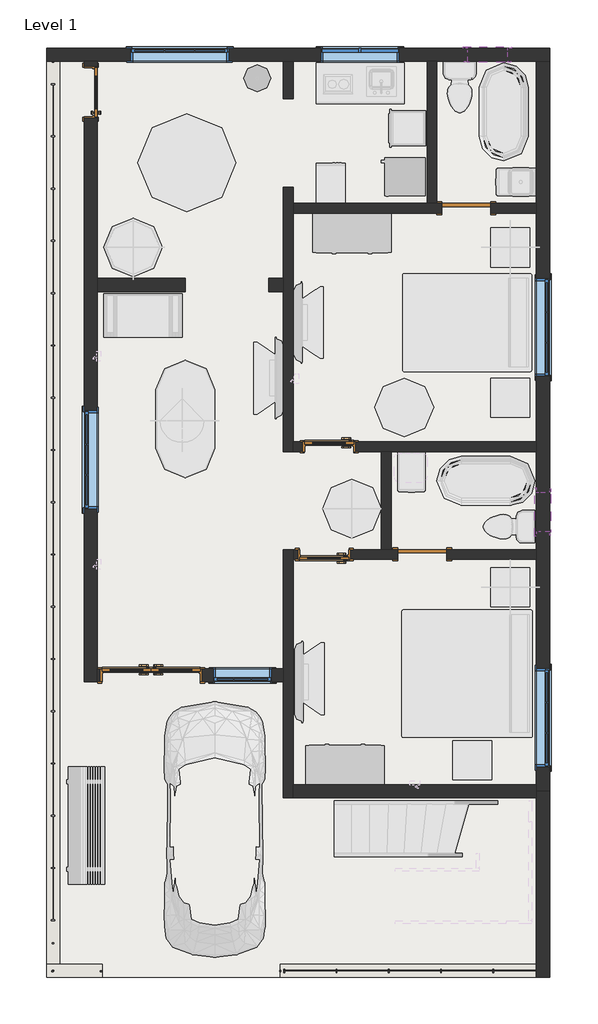
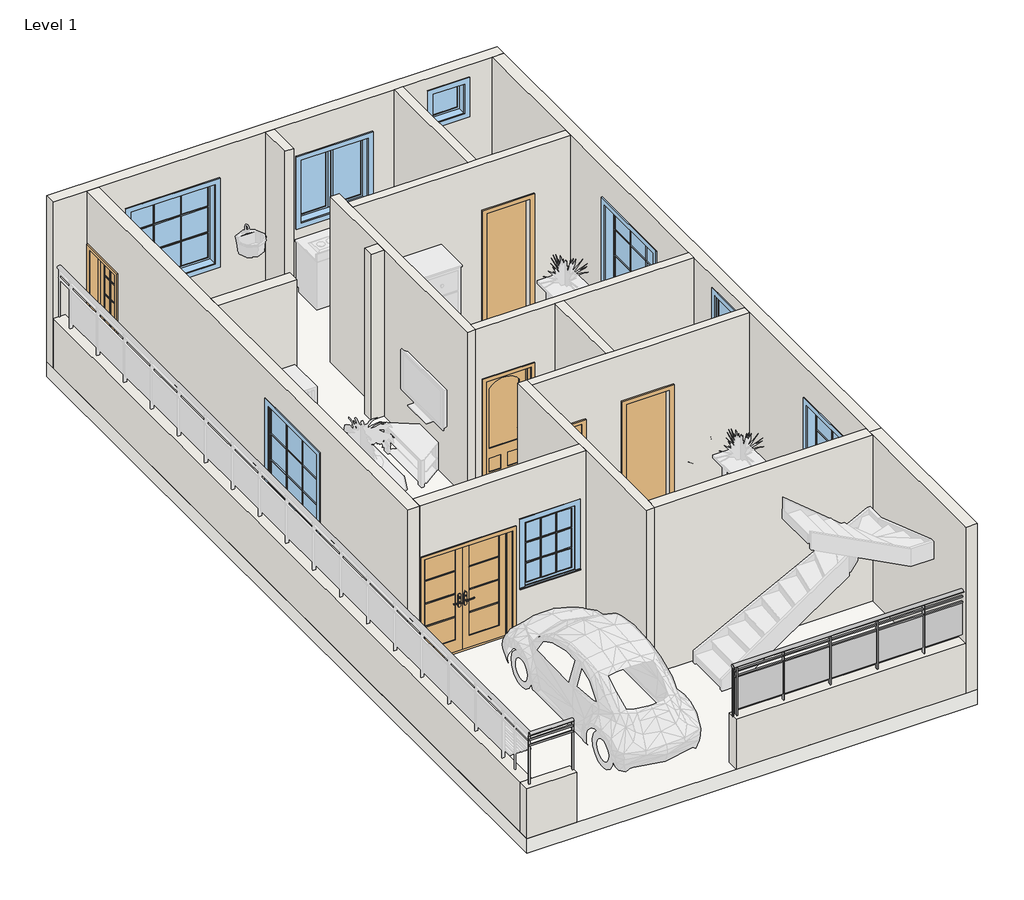
# One storey, part 1 of 2: 19 walls, 8 windows, 6 doors, 2 railings, 1 slab.
"""IFC4 building model written with IfcOpenShell, lengths in millimetres."""

from ifc_helpers import new_model, si_unit, point, frame, origin, origin_with_axes, place, context, project, spatial, polyline, ellipse_curve, trimmed, outline, extrude, faceted_brep, transform, mapped, element, save
from ifc_brep_helpers import plane_surface, extruded_surface, advanced_brep
from components import door_4b146b56, door_14b9be53, door_b03bd389, door_d788789e, door_e2b13fe9, window_29c06734, window_8901c6e2, window_0862ab64, window_e41d21a6

model = new_model("IFC4")

# Units and contexts
model_context = context("Model", 3, world=origin())
ifc_project = project(units=[si_unit("LENGTHUNIT", "METRE", prefix="MILLI")], contexts=[model_context])

# Site, building, storey
site = spatial("IfcSite", under=ifc_project)
building = spatial("IfcBuilding", under=site)
storey = spatial("IfcBuildingStorey", under=building, Name="Level 1", Elevation=0.0)

# Doors
placement = place(None, origin())
door_shape = door_4b146b56(model_context)
element("IfcDoor", 1, ObjectType="30\" x 80\"", at=placement, inside=storey, context=model_context, shape_type="MappedRepresentation", body=[
    mapped(door_shape, transform((-1899.3247449, 6788.0508877, 0.0), x_axis=(1.0, 0.0, 0.0), y_axis=(0.0, 1.0, 0.0), z_axis=(0.0, 0.0, 1.0))),
])
door_2_shape = door_14b9be53(model_context)
element("IfcDoor", 2, ObjectType="30\" x 80\"", at=placement, inside=storey, context=model_context, shape_type="MappedRepresentation", body=[
    mapped(door_2_shape, transform((-1823.1247449, 8470.8008877, 0.0), x_axis=(1.0, 0.0, 0.0), y_axis=(0.0, 1.0, 0.0), z_axis=(0.0, 0.0, 1.0))),
])
door_3_shape = door_b03bd389(model_context)
element("IfcDoor", 3, ObjectType="Door-Exterior-Double-Full Glass-Wood_Clad : 60\" x 80\"", at=placement, inside=storey, context=model_context, shape_type="MappedRepresentation", body=[
    mapped(door_3_shape, transform((-4591.7247449, 4914.8008877, 0.0), x_axis=(1.0, 0.0, 0.0), y_axis=(0.0, 1.0, 0.0), z_axis=(0.0, 0.0, 1.0))),
])
door_4_shape = door_d788789e(model_context)
element("IfcDoor", 4, ObjectType="Door-Interior-Single-Full Glass-Wood : 30\" x 80\"", at=placement, inside=storey, context=model_context, shape_type="MappedRepresentation", body=[
    mapped(door_4_shape, transform((-5528.3497449, 13979.4258877, 0.0), x_axis=(0.0, 1.0, 0.0), y_axis=(-1.0, 0.0, 0.0), z_axis=(0.0, 0.0, 1.0))),
])
door_5_shape = door_e2b13fe9(model_context)
element("IfcDoor", 5, ObjectType="Single-Flush : 30\" x 84\"", at=placement, inside=storey, context=model_context, shape_type="MappedRepresentation", body=[
    mapped(door_5_shape, transform((-375.3247449, 6791.2258877, 0.0), x_axis=(-1.0, 0.0, 0.0), y_axis=(0.0, -1.0, 0.0), z_axis=(0.0, 0.0, 1.0))),
])
element("IfcDoor", 6, ObjectType="Single-Flush : 30\" x 84\"", at=placement, inside=storey, context=model_context, shape_type="MappedRepresentation", body=[
    mapped(door_5_shape, transform((310.4752551, 12176.0258877, 0.0), x_axis=(-1.0, 0.0, 0.0), y_axis=(0.0, -1.0, 0.0), z_axis=(0.0, 0.0, 1.0))),
])

# Railings
element("IfcRailing", 7, ObjectType="Glass Panel - Bottom Fill", at=placement, inside=storey, context=model_context, shape_type="SolidModel", body=[
    advanced_brep(
    [(-2585.1247449, 352.3258877, 1828.8), (-2585.1247449, 276.1258877, 1828.8), (1605.8752551, 352.3258877, 1828.8), (1605.8752551, 276.1258877, 1828.8)],
    [
        (0, 1, ellipse_curve(frame((-2585.1247449, 314.2258877, 1828.8), z_axis=(-1.0, 0.0, 0.0), x_axis=(0.0, -1.0, 0.0)), 38.1, 28.575)),
        (1, 0, ellipse_curve(frame((-2585.1247449, 314.2258877, 1828.8), z_axis=(-1.0, 0.0, 0.0), x_axis=(0.0, -1.0, 0.0)), 38.1, 28.575)),
        (2, 3, ellipse_curve(frame((1605.8752551, 314.2258877, 1828.8), z_axis=(1.0, 0.0, 0.0), x_axis=(0.0, -1.0, 0.0)), 38.1, 28.575)),
        (3, 2, ellipse_curve(frame((1605.8752551, 314.2258877, 1828.8), z_axis=(1.0, 0.0, 0.0), x_axis=(0.0, -1.0, 0.0)), 38.1, 28.575)),
        (0, 2),
        (3, 1),
    ],
    [
        plane_surface(frame((-2585.1247449, 314.2258877, 1828.8), z_axis=(-1.0, 0.0, 0.0), x_axis=(0.0, 1.0, 0.0))),
        plane_surface(frame((1605.8752551, 314.2258877, 1828.8), z_axis=(1.0, 0.0, 0.0), x_axis=(0.0, 1.0, 0.0))),
        extruded_surface(trimmed(ellipse_curve(frame((1605.8752551, 314.2258877, 1828.8), z_axis=(-1.0, 0.0, 0.0), x_axis=(0.0, -1.0, 0.0)), 38.1, 28.575), [point((1605.8752551, 352.3258877, 1828.8))], [point((1605.8752551, 276.1258877, 1828.8))], True, "CARTESIAN"), (-4191.0, 0.0, 0.0), 4191.0),
        extruded_surface(trimmed(ellipse_curve(frame((1605.8752551, 314.2258877, 1828.8), z_axis=(-1.0, 0.0, 0.0), x_axis=(0.0, -1.0, 0.0)), 38.1, 28.575), [point((1605.8752551, 276.1258877, 1828.8))], [point((1605.8752551, 352.3258877, 1828.8))], True, "CARTESIAN"), (-4191.0, 0.0, 0.0), 4191.0),
    ],
    [
        (0, [[1, 2]]),
        (1, [[3, 4]]),
        (2, [[-1, 5, -4, 6]]),
        (3, [[-2, -6, -3, -5]]),
    ],
),
    extrude(outline(polyline([(-2585.1247449, 301.5258877), (-2585.1247449, 326.9258877), (1605.8752551, 326.9258877), (1605.8752551, 301.5258877), (-2585.1247449, 301.5258877)])), frame((0.0, 0.0, 1714.5), z_axis=(0.0, 0.0, 1.0), x_axis=(1.0, 0.0, 0.0)), (0.0, 0.0, 1.0), 25.4),
    extrude(outline(polyline([(-2585.1247449, 301.5258877), (-2585.1247449, 326.9258877), (1605.8752551, 326.9258877), (1605.8752551, 301.5258877), (-2585.1247449, 301.5258877)])), frame((0.0, 0.0, 1612.9), z_axis=(0.0, 0.0, 1.0), x_axis=(1.0, 0.0, 0.0)), (0.0, 0.0, 1.0), 25.4),
    extrude(outline(polyline([(1536.0252551, 288.8258877), (1536.0252551, 339.6258877), (1548.7252551, 339.6258877), (1548.7252551, 288.8258877), (1536.0252551, 288.8258877)])), frame((0.0, 0.0, 914.4), z_axis=(0.0, 0.0, 1.0), x_axis=(1.0, 0.0, 0.0)), (0.0, 0.0, 1.0), 885.6788223),
    extrude(outline(polyline([(729.5752551, 320.7610448), (1542.3752551, 320.7610448), (1542.3752551, 314.4110448), (729.5752551, 314.4110448), (729.5752551, 320.7610448)])), frame((0.0, 0.0, 1016.0), z_axis=(0.0, 0.0, 1.0), x_axis=(1.0, 0.0, 0.0)), (0.0, 0.0, 1.0), 596.9),
    extrude(outline(polyline([(723.2252551, 288.8258877), (723.2252551, 339.6258877), (735.9252551, 339.6258877), (735.9252551, 288.8258877), (723.2252551, 288.8258877)])), frame((0.0, 0.0, 914.4), z_axis=(0.0, 0.0, 1.0), x_axis=(1.0, 0.0, 0.0)), (0.0, 0.0, 1.0), 885.6788223),
    extrude(outline(polyline([(-83.2247449, 320.7610448), (729.5752551, 320.7610448), (729.5752551, 314.4110448), (-83.2247449, 314.4110448), (-83.2247449, 320.7610448)])), frame((0.0, 0.0, 1016.0), z_axis=(0.0, 0.0, 1.0), x_axis=(1.0, 0.0, 0.0)), (0.0, 0.0, 1.0), 596.9),
    extrude(outline(polyline([(-89.5747449, 288.8258877), (-89.5747449, 339.6258877), (-76.8747449, 339.6258877), (-76.8747449, 288.8258877), (-89.5747449, 288.8258877)])), frame((0.0, 0.0, 914.4), z_axis=(0.0, 0.0, 1.0), x_axis=(1.0, 0.0, 0.0)), (0.0, 0.0, 1.0), 885.6788223),
    extrude(outline(polyline([(-896.0247449, 320.7610448), (-83.2247449, 320.7610448), (-83.2247449, 314.4110448), (-896.0247449, 314.4110448), (-896.0247449, 320.7610448)])), frame((0.0, 0.0, 1016.0), z_axis=(0.0, 0.0, 1.0), x_axis=(1.0, 0.0, 0.0)), (0.0, 0.0, 1.0), 596.9),
    extrude(outline(polyline([(-902.3747449, 288.8258877), (-902.3747449, 339.6258877), (-889.6747449, 339.6258877), (-889.6747449, 288.8258877), (-902.3747449, 288.8258877)])), frame((0.0, 0.0, 914.4), z_axis=(0.0, 0.0, 1.0), x_axis=(1.0, 0.0, 0.0)), (0.0, 0.0, 1.0), 885.6788223),
    extrude(outline(polyline([(-1708.8247449, 320.7610448), (-896.0247449, 320.7610448), (-896.0247449, 314.4110448), (-1708.8247449, 314.4110448), (-1708.8247449, 320.7610448)])), frame((0.0, 0.0, 1016.0), z_axis=(0.0, 0.0, 1.0), x_axis=(1.0, 0.0, 0.0)), (0.0, 0.0, 1.0), 596.9),
    extrude(outline(polyline([(-1715.1747449, 288.8258877), (-1715.1747449, 339.6258877), (-1702.4747449, 339.6258877), (-1702.4747449, 288.8258877), (-1715.1747449, 288.8258877)])), frame((0.0, 0.0, 914.4), z_axis=(0.0, 0.0, 1.0), x_axis=(1.0, 0.0, 0.0)), (0.0, 0.0, 1.0), 885.6788223),
    extrude(outline(polyline([(-2521.6247449, 320.7610448), (-1708.8247449, 320.7610448), (-1708.8247449, 314.4110448), (-2521.6247449, 314.4110448), (-2521.6247449, 320.7610448)])), frame((0.0, 0.0, 1016.0), z_axis=(0.0, 0.0, 1.0), x_axis=(1.0, 0.0, 0.0)), (0.0, 0.0, 1.0), 596.9),
    extrude(outline(polyline([(-2527.9747449, 288.8258877), (-2527.9747449, 339.6258877), (-2515.2747449, 339.6258877), (-2515.2747449, 288.8258877), (-2527.9747449, 288.8258877)])), frame((0.0, 0.0, 914.4), z_axis=(0.0, 0.0, 1.0), x_axis=(1.0, 0.0, 0.0)), (0.0, 0.0, 1.0), 885.6788223),
    extrude(outline(polyline([(1593.1752551, 304.7008877), (1593.1752551, 323.7508877), (1612.2252551, 323.7508877), (1612.2252551, 304.7008877), (1593.1752551, 304.7008877)])), frame((0.0, 0.0, 914.4), z_axis=(0.0, 0.0, 1.0), x_axis=(1.0, 0.0, 0.0)), (0.0, 0.0, 1.0), 885.6788223),
    extrude(outline(polyline([(-2591.4747449, 304.7008877), (-2591.4747449, 323.7508877), (-2572.4247449, 323.7508877), (-2572.4247449, 304.7008877), (-2591.4747449, 304.7008877)])), frame((0.0, 0.0, 914.4), z_axis=(0.0, 0.0, 1.0), x_axis=(1.0, 0.0, 0.0)), (0.0, 0.0, 1.0), 885.6788223),
])
element("IfcRailing", 8, ObjectType="Glass Panel - Bottom Fill", at=placement, inside=storey, context=model_context, shape_type="SolidModel", body=[
    advanced_brep(
    [(-6128.4247449, 345.9758877, 1828.8), (-6128.4247449, 269.7758877, 1828.8), (-5366.4247449, 345.9758877, 1828.8), (-5366.4247449, 269.7758877, 1828.8)],
    [
        (0, 1, ellipse_curve(frame((-6128.4247449, 307.8758877, 1828.8), z_axis=(-1.0, 0.0, 0.0), x_axis=(0.0, -1.0, 0.0)), 38.1, 28.575)),
        (1, 0, ellipse_curve(frame((-6128.4247449, 307.8758877, 1828.8), z_axis=(-1.0, 0.0, 0.0), x_axis=(0.0, -1.0, 0.0)), 38.1, 28.575)),
        (2, 3, ellipse_curve(frame((-5366.4247449, 307.8758877, 1828.8), z_axis=(1.0, 0.0, 0.0), x_axis=(0.0, -1.0, 0.0)), 38.1, 28.575)),
        (3, 2, ellipse_curve(frame((-5366.4247449, 307.8758877, 1828.8), z_axis=(1.0, 0.0, 0.0), x_axis=(0.0, -1.0, 0.0)), 38.1, 28.575)),
        (0, 2),
        (3, 1),
    ],
    [
        plane_surface(frame((-6128.4247449, 307.8758877, 1828.8), z_axis=(-1.0, 0.0, 0.0), x_axis=(0.0, 1.0, 0.0))),
        plane_surface(frame((-5366.4247449, 307.8758877, 1828.8), z_axis=(1.0, 0.0, 0.0), x_axis=(0.0, 1.0, 0.0))),
        extruded_surface(trimmed(ellipse_curve(frame((-5366.4247449, 307.8758877, 1828.8), z_axis=(-1.0, 0.0, 0.0), x_axis=(0.0, -1.0, 0.0)), 38.1, 28.575), [point((-5366.4247449, 345.9758877, 1828.8))], [point((-5366.4247449, 269.7758877, 1828.8))], True, "CARTESIAN"), (-762.0, 0.0, 0.0), 762.0),
        extruded_surface(trimmed(ellipse_curve(frame((-5366.4247449, 307.8758877, 1828.8), z_axis=(-1.0, 0.0, 0.0), x_axis=(0.0, -1.0, 0.0)), 38.1, 28.575), [point((-5366.4247449, 269.7758877, 1828.8))], [point((-5366.4247449, 345.9758877, 1828.8))], True, "CARTESIAN"), (-762.0, 0.0, 0.0), 762.0),
    ],
    [
        (0, [[1, 2]]),
        (1, [[3, 4]]),
        (2, [[-1, 5, -4, 6]]),
        (3, [[-2, -6, -3, -5]]),
    ],
),
    extrude(outline(polyline([(-6128.4247449, 295.1758877), (-6128.4247449, 320.5758877), (-5366.4247449, 320.5758877), (-5366.4247449, 295.1758877), (-6128.4247449, 295.1758877)])), frame((0.0, 0.0, 1714.5), z_axis=(0.0, 0.0, 1.0), x_axis=(1.0, 0.0, 0.0)), (0.0, 0.0, 1.0), 25.4),
    extrude(outline(polyline([(-6128.4247449, 295.1758877), (-6128.4247449, 320.5758877), (-5366.4247449, 320.5758877), (-5366.4247449, 295.1758877), (-6128.4247449, 295.1758877)])), frame((0.0, 0.0, 1612.9), z_axis=(0.0, 0.0, 1.0), x_axis=(1.0, 0.0, 0.0)), (0.0, 0.0, 1.0), 25.4),
    extrude(outline(polyline([(-5379.1247449, 298.3508877), (-5379.1247449, 317.4008877), (-5360.0747449, 317.4008877), (-5360.0747449, 298.3508877), (-5379.1247449, 298.3508877)])), frame((0.0, 0.0, 914.4), z_axis=(0.0, 0.0, 1.0), x_axis=(1.0, 0.0, 0.0)), (0.0, 0.0, 1.0), 885.6788223),
    extrude(outline(polyline([(-6134.7747449, 298.3508877), (-6134.7747449, 317.4008877), (-6115.7247449, 317.4008877), (-6115.7247449, 298.3508877), (-6134.7747449, 298.3508877)])), frame((0.0, 0.0, 914.4), z_axis=(0.0, 0.0, 1.0), x_axis=(1.0, 0.0, 0.0)), (0.0, 0.0, 1.0), 885.6788223),
])

# Slab
element("IfcSlab", 9, ObjectType="Wood Joist 10\" - Ceramic Tile", at=placement, inside=storey, context=model_context, shape_type="SweptSolid", body=[
    extrude(outline(polyline([(1605.8752551, 14665.2258877), (1605.8752551, 212.6258877), (-6217.3247449, 212.6258877), (-6217.3247449, 14665.2258877), (1605.8752551, 14665.2258877)])), frame((0.0, 0.0, -273.05), z_axis=(0.0, 0.0, 1.0), x_axis=(1.0, 0.0, 0.0)), (0.0, 0.0, 1.0), 273.05),
])

# Walls
element("IfcWall", 10, ObjectType="Generic - 8\"", at=placement, inside=storey, context=model_context, shape_type="Brep", body=[
    faceted_brep([(-6217.3247449, 14462.0258877, 0.0), (-6014.1247449, 14462.0258877, 0.0), (-5633.1247449, 14462.0258877, 0.0), (-5429.9247449, 14462.0258877, 0.0), (-2534.3247449, 14462.0258877, 0.0), (-2381.9247449, 14462.0258877, 0.0), (-299.1247449, 14462.0258877, 0.0), (-146.7247449, 14462.0258877, 0.0), (1402.6752551, 14462.0258877, 0.0), (1605.8752551, 14462.0258877, 0.0), (1605.8752551, 14462.0258877, 3048.0), (1402.6752551, 14462.0258877, 3048.0), (-146.7247449, 14462.0258877, 3048.0), (-299.1247449, 14462.0258877, 3048.0), (-2381.9247449, 14462.0258877, 3048.0), (-2534.3247449, 14462.0258877, 3048.0), (-5429.9247449, 14462.0258877, 3048.0), (-5633.1247449, 14462.0258877, 3048.0), (-6217.3247449, 14462.0258877, 3048.0), (-6217.3247449, 14462.0258877, 914.4), (-3385.2247449, 14462.0258877, 2438.4), (-3385.2247449, 14462.0258877, 914.4), (-4909.2247449, 14462.0258877, 914.4), (-4909.2247449, 14462.0258877, 2438.4), (-730.9247449, 14462.0258877, 2362.2), (-730.9247449, 14462.0258877, 1143.0), (-1950.1247449, 14462.0258877, 1143.0), (-1950.1247449, 14462.0258877, 2362.2), (945.4752551, 14462.0258877, 2768.6), (945.4752551, 14462.0258877, 2159.0), (335.8752551, 14462.0258877, 2159.0), (335.8752551, 14462.0258877, 2768.6), (-6217.3247449, 14665.2258877, 0.0), (-6217.3247449, 14665.2258877, 3048.0), (1605.8752551, 14665.2258877, 3048.0), (1605.8752551, 14665.2258877, 0.0), (-3385.2247449, 14665.2258877, 2438.4), (-4909.2247449, 14665.2258877, 2438.4), (-4909.2247449, 14665.2258877, 914.4), (-3385.2247449, 14665.2258877, 914.4), (-730.9247449, 14665.2258877, 2362.2), (-1950.1247449, 14665.2258877, 2362.2), (-1950.1247449, 14665.2258877, 1143.0), (-730.9247449, 14665.2258877, 1143.0), (945.4752551, 14665.2258877, 2768.6), (335.8752551, 14665.2258877, 2768.6), (335.8752551, 14665.2258877, 2159.0), (945.4752551, 14665.2258877, 2159.0)], [[[0, 1, 2, 3, 4, 5, 6, 7, 8, 9, 10, 11, 12, 13, 14, 15, 16, 17, 18, 19], [20, 21, 22, 23], [24, 25, 26, 27], [28, 29, 30, 31]], [[32, 33, 34, 35], [36, 37, 38, 39], [40, 41, 42, 43], [44, 45, 46, 47]], [[9, 8, 7, 6, 5, 4, 3, 2, 1, 0, 32, 35]], [[10, 9, 35, 34]], [[0, 19, 18, 33, 32]], [[18, 17, 16, 15, 14, 13, 12, 11, 10, 34, 33]], [[21, 20, 36, 39]], [[22, 21, 39, 38]], [[23, 22, 38, 37]], [[20, 23, 37, 36]], [[25, 24, 40, 43]], [[26, 25, 43, 42]], [[27, 26, 42, 41]], [[24, 27, 41, 40]], [[29, 28, 44, 47]], [[30, 29, 47, 46]], [[31, 30, 46, 45]], [[28, 31, 45, 44]]]),
])
element("IfcWall", 11, ObjectType="Generic - 8\"", at=placement, inside=storey, context=model_context, shape_type="Brep", body=[
    faceted_brep([(1402.6752551, 14462.0258877, 0.0), (1402.6752551, 12252.2258877, 0.0), (1402.6752551, 12099.8258877, 0.0), (1402.6752551, 8543.8258877, 0.0), (1402.6752551, 8391.4258877, 0.0), (1402.6752551, 6867.4258877, 0.0), (1402.6752551, 6715.0258877, 0.0), (1402.6752551, 3209.8258877, 0.0), (1402.6752551, 3108.2258877, 0.0), (1402.6752551, 3108.2258877, 3048.0), (1402.6752551, 3209.8258877, 3048.0), (1402.6752551, 6715.0258877, 3048.0), (1402.6752551, 6867.4258877, 3048.0), (1402.6752551, 8391.4258877, 3048.0), (1402.6752551, 8543.8258877, 3048.0), (1402.6752551, 12099.8258877, 3048.0), (1402.6752551, 12252.2258877, 3048.0), (1402.6752551, 14462.0258877, 3048.0), (1402.6752551, 9559.8258877, 2438.4), (1402.6752551, 9559.8258877, 914.4), (1402.6752551, 11083.8258877, 914.4), (1402.6752551, 11083.8258877, 2438.4), (1402.6752551, 3489.2258877, 2438.4), (1402.6752551, 3489.2258877, 914.4), (1402.6752551, 5013.2258877, 914.4), (1402.6752551, 5013.2258877, 2438.4), (1402.6752551, 7756.4258877, 2768.6), (1402.6752551, 7146.8258877, 2768.6), (1402.6752551, 7146.8258877, 2159.0), (1402.6752551, 7756.4258877, 2159.0), (1605.8752551, 14462.0258877, 0.0), (1605.8752551, 14462.0258877, 3048.0), (1605.8752551, 3108.2258877, 3048.0), (1605.8752551, 3108.2258877, 0.0), (1605.8752551, 9559.8258877, 2438.4), (1605.8752551, 11083.8258877, 2438.4), (1605.8752551, 11083.8258877, 914.4), (1605.8752551, 9559.8258877, 914.4), (1605.8752551, 3489.2258877, 2438.4), (1605.8752551, 5013.2258877, 2438.4), (1605.8752551, 5013.2258877, 914.4), (1605.8752551, 3489.2258877, 914.4), (1605.8752551, 7756.4258877, 2768.6), (1605.8752551, 7756.4258877, 2159.0), (1605.8752551, 7146.8258877, 2159.0), (1605.8752551, 7146.8258877, 2768.6)], [[[0, 1, 2, 3, 4, 5, 6, 7, 8, 9, 10, 11, 12, 13, 14, 15, 16, 17], [18, 19, 20, 21], [22, 23, 24, 25], [26, 27, 28, 29]], [[30, 31, 32, 33], [34, 35, 36, 37], [38, 39, 40, 41], [42, 43, 44, 45]], [[8, 7, 6, 5, 4, 3, 2, 1, 0, 30, 33]], [[9, 8, 33, 32]], [[0, 17, 31, 30]], [[17, 16, 15, 14, 13, 12, 11, 10, 9, 32, 31]], [[19, 18, 34, 37]], [[20, 19, 37, 36]], [[21, 20, 36, 35]], [[18, 21, 35, 34]], [[23, 22, 38, 41]], [[24, 23, 41, 40]], [[25, 24, 40, 39]], [[22, 25, 39, 38]], [[43, 42, 26, 29]], [[44, 43, 29, 28]], [[45, 44, 28, 27]], [[42, 45, 27, 26]]]),
])
element("IfcWall", 12, ObjectType="Generic - 8\"", at=placement, inside=storey, context=model_context, shape_type="Brep", body=[
    faceted_brep([(-5633.1247449, 14462.0258877, 3048.0), (-5633.1247449, 14462.0258877, 0.0), (-5633.1247449, 14385.8258877, 0.0), (-5633.1247449, 14385.8258877, 2057.4), (-5633.1247449, 13573.0258877, 2057.4), (-5633.1247449, 13573.0258877, 0.0), (-5633.1247449, 4810.0258877, 0.0), (-5633.1247449, 4810.0258877, 3048.0), (-5633.1247449, 9026.4258877, 2438.4), (-5633.1247449, 7502.4258877, 2438.4), (-5633.1247449, 7502.4258877, 914.4), (-5633.1247449, 9026.4258877, 914.4), (-5429.9247449, 14462.0258877, 0.0), (-5429.9247449, 14462.0258877, 3048.0), (-5429.9247449, 11083.8258877, 3048.0), (-5429.9247449, 10880.6258877, 3048.0), (-5429.9247449, 5013.2258877, 3048.0), (-5429.9247449, 4810.0258877, 3048.0), (-5429.9247449, 4810.0258877, 0.0), (-5429.9247449, 5013.2258877, 0.0), (-5429.9247449, 10880.6258877, 0.0), (-5429.9247449, 11083.8258877, 0.0), (-5429.9247449, 13573.0258877, 0.0), (-5429.9247449, 13573.0258877, 2057.4), (-5429.9247449, 14385.8258877, 2057.4), (-5429.9247449, 14385.8258877, 0.0), (-5429.9247449, 9026.4258877, 2438.4), (-5429.9247449, 9026.4258877, 914.4), (-5429.9247449, 7502.4258877, 914.4), (-5429.9247449, 7502.4258877, 2438.4)], [[[0, 1, 2, 3, 4, 5, 6, 7], [8, 9, 10, 11]], [[12, 13, 14, 15, 16, 17, 18, 19, 20, 21, 22, 23, 24, 25], [26, 27, 28, 29]], [[1, 12, 25, 2]], [[18, 6, 5, 22, 21, 20, 19]], [[1, 0, 13, 12]], [[7, 6, 18, 17]], [[0, 7, 17, 16, 15, 14, 13]], [[27, 26, 8, 11]], [[28, 27, 11, 10]], [[29, 28, 10, 9]], [[26, 29, 9, 8]], [[24, 3, 2, 25]], [[3, 24, 23, 4]], [[4, 23, 22, 5]]]),
])
element("IfcWall", 13, ObjectType="Generic - 8\"", at=placement, inside=storey, context=model_context, shape_type="Brep", body=[
    faceted_brep([(-2381.9247449, 3006.6258877, 0.0), (1402.6752551, 3006.6258877, 0.0), (1402.6752551, 3006.6258877, 3048.0), (-2381.9247449, 3006.6258877, 3048.0), (-2381.9247449, 3209.8258877, 0.0), (-2381.9247449, 3209.8258877, 3048.0), (1402.6752551, 3209.8258877, 3048.0), (1402.6752551, 3209.8258877, 0.0), (1402.6752551, 3108.2258877, 0.0), (1402.6752551, 3108.2258877, 3048.0)], [[[0, 1, 2, 3]], [[4, 5, 6, 7]], [[1, 0, 4, 7, 8]], [[0, 3, 5, 4]], [[3, 2, 9, 6, 5]], [[2, 1, 8, 7, 6, 9]]]),
])
element("IfcWall", 14, ObjectType="Generic - 8\"", at=placement, inside=storey, context=model_context, shape_type="SweptSolid", body=[
    extrude(outline(polyline([(0.0, -2534.3247449), (3048.0, -2534.3247449), (3048.0, -5429.9247449), (0.0, -5429.9247449), (0.0, -5379.1247449), (2057.4, -5379.1247449), (2057.4, -3804.3247449), (0.0, -3804.3247449), (0.0, -2534.3247449)]), holes=[polyline([(2133.6, -3626.5247449), (2133.6, -2712.1247449), (914.4, -2712.1247449), (914.4, -3626.5247449), (2133.6, -3626.5247449)])]), frame((0.0, 4810.0258877, 0.0), z_axis=(0.0, 1.0, 0.0), x_axis=(0.0, 0.0, 1.0)), (0.0, 0.0, 1.0), 203.2),
])
element("IfcWall", 15, ObjectType="Generic - 8\"", at=placement, inside=storey, context=model_context, shape_type="Brep", body=[
    faceted_brep([(1402.6752551, 3108.2258877, 0.0), (1402.6752551, 3006.6258877, 0.0), (1402.6752551, 415.8258877, 0.0), (1402.6752551, 212.6258877, 0.0), (1402.6752551, 212.6258877, 914.4), (1402.6752551, 212.6258877, 3048.0), (1402.6752551, 3006.6258877, 3048.0), (1402.6752551, 3108.2258877, 3048.0), (1605.8752551, 3108.2258877, 0.0), (1605.8752551, 3108.2258877, 3048.0), (1605.8752551, 212.6258877, 3048.0), (1605.8752551, 212.6258877, 0.0)], [[[0, 1, 2, 3, 4, 5, 6, 7]], [[8, 9, 10, 11]], [[3, 2, 1, 0, 8, 11]], [[7, 6, 5, 10, 9]], [[0, 7, 9, 8]], [[5, 4, 3, 11, 10]]]),
])
element("IfcWall", 16, ObjectType="Generic - 8\"", at=placement, inside=storey, context=model_context, shape_type="SweptSolid", body=[
    extrude(outline(polyline([(-2762.9247449, 11083.8258877), (-2534.3247449, 11083.8258877), (-2534.3247449, 10880.6258877), (-2762.9247449, 10880.6258877), (-2762.9247449, 11083.8258877)])), origin_with_axes(), (0.0, 0.0, 1.0), 3048.0),
])
element("IfcWall", 17, ObjectType="Generic - 8\"", at=placement, inside=storey, context=model_context, shape_type="SweptSolid", body=[
    extrude(outline(polyline([(-5429.9247449, 11083.8258877), (-4058.3247449, 11083.8258877), (-4058.3247449, 10880.6258877), (-5429.9247449, 10880.6258877), (-5429.9247449, 11083.8258877)])), origin_with_axes(), (0.0, 0.0, 1.0), 3048.0),
])
element("IfcWall", 18, ObjectType="inner wall", at=placement, inside=storey, context=model_context, shape_type="SweptSolid", body=[
    extrude(outline(polyline([(-2534.3247449, 13877.8258877), (-2534.3247449, 14462.0258877), (-2381.9247449, 14462.0258877), (-2381.9247449, 13877.8258877), (-2534.3247449, 13877.8258877)])), origin_with_axes(), (0.0, 0.0, 1.0), 3048.0),
])
element("IfcWall", 19, ObjectType="inner wall", at=placement, inside=storey, context=model_context, shape_type="Brep", body=[
    faceted_brep([(1402.6752551, 6867.4258877, 3048.0), (1402.6752551, 6867.4258877, 0.0), (5.6752551, 6867.4258877, 0.0), (5.6752551, 6867.4258877, 2133.6), (-756.3247449, 6867.4258877, 2133.6), (-756.3247449, 6867.4258877, 0.0), (-857.9247449, 6867.4258877, 0.0), (-1010.3247449, 6867.4258877, 0.0), (-1492.9247449, 6867.4258877, 0.0), (-1492.9247449, 6867.4258877, 2057.4), (-2305.7247449, 6867.4258877, 2057.4), (-2305.7247449, 6867.4258877, 0.0), (-2381.9247449, 6867.4258877, 0.0), (-2381.9247449, 6867.4258877, 3048.0), (-1010.3247449, 6867.4258877, 3048.0), (-857.9247449, 6867.4258877, 3048.0), (1402.6752551, 6715.0258877, 0.0), (1402.6752551, 6715.0258877, 3048.0), (-2381.9247449, 6715.0258877, 3048.0), (-2381.9247449, 6715.0258877, 0.0), (-2305.7247449, 6715.0258877, 0.0), (-2305.7247449, 6715.0258877, 2057.4), (-1492.9247449, 6715.0258877, 2057.4), (-1492.9247449, 6715.0258877, 0.0), (-756.3247449, 6715.0258877, 0.0), (-756.3247449, 6715.0258877, 2133.6), (5.6752551, 6715.0258877, 2133.6), (5.6752551, 6715.0258877, 0.0)], [[[0, 1, 2, 3, 4, 5, 6, 7, 8, 9, 10, 11, 12, 13, 14, 15]], [[16, 17, 18, 19, 20, 21, 22, 23, 24, 25, 26, 27]], [[1, 16, 27, 2]], [[19, 12, 11, 20]], [[5, 24, 23, 8, 7, 6]], [[1, 0, 17, 16]], [[0, 15, 14, 13, 18, 17]], [[13, 12, 19, 18]], [[25, 24, 5, 4]], [[26, 25, 4, 3]], [[27, 26, 3, 2]], [[22, 9, 8, 23]], [[9, 22, 21, 10]], [[10, 21, 20, 11]]]),
])
element("IfcWall", 20, ObjectType="inner wall", at=placement, inside=storey, context=model_context, shape_type="Brep", body=[
    faceted_brep([(1402.6752551, 8543.8258877, 3048.0), (1402.6752551, 8543.8258877, 0.0), (-1416.7247449, 8543.8258877, 0.0), (-1416.7247449, 8543.8258877, 2057.4), (-2229.5247449, 8543.8258877, 2057.4), (-2229.5247449, 8543.8258877, 0.0), (-2381.9247449, 8543.8258877, 0.0), (-2381.9247449, 8543.8258877, 3048.0), (1402.6752551, 8391.4258877, 0.0), (1402.6752551, 8391.4258877, 3048.0), (-857.9247449, 8391.4258877, 3048.0), (-1010.3247449, 8391.4258877, 3048.0), (-2381.9247449, 8391.4258877, 3048.0), (-2381.9247449, 8391.4258877, 0.0), (-2229.5247449, 8391.4258877, 0.0), (-2229.5247449, 8391.4258877, 2057.4), (-1416.7247449, 8391.4258877, 2057.4), (-1416.7247449, 8391.4258877, 0.0), (-1010.3247449, 8391.4258877, 0.0), (-857.9247449, 8391.4258877, 0.0)], [[[0, 1, 2, 3, 4, 5, 6, 7]], [[8, 9, 10, 11, 12, 13, 14, 15, 16, 17, 18, 19]], [[1, 8, 19, 18, 17, 2]], [[13, 6, 5, 14]], [[1, 0, 9, 8]], [[0, 7, 12, 11, 10, 9]], [[7, 6, 13, 12]], [[16, 3, 2, 17]], [[3, 16, 15, 4]], [[4, 15, 14, 5]]]),
])
element("IfcWall", 21, ObjectType="inner wall", at=placement, inside=storey, context=model_context, shape_type="SweptSolid", body=[
    extrude(outline(polyline([(-1010.3247449, 6867.4258877), (-1010.3247449, 8391.4258877), (-857.9247449, 8391.4258877), (-857.9247449, 6867.4258877), (-1010.3247449, 6867.4258877)])), origin_with_axes(), (0.0, 0.0, 1.0), 3048.0),
])
element("IfcWall", 22, ObjectType="inner wall", at=placement, inside=storey, context=model_context, shape_type="Brep", body=[
    faceted_brep([(-70.5247449, 12252.2258877, 2133.6), (-70.5247449, 12252.2258877, 0.0), (-146.7247449, 12252.2258877, 0.0), (-299.1247449, 12252.2258877, 0.0), (-2381.9247449, 12252.2258877, 0.0), (-2381.9247449, 12252.2258877, 3048.0), (-299.1247449, 12252.2258877, 3048.0), (-146.7247449, 12252.2258877, 3048.0), (1402.6752551, 12252.2258877, 3048.0), (1402.6752551, 12252.2258877, 0.0), (691.4752551, 12252.2258877, 0.0), (691.4752551, 12252.2258877, 2133.6), (-2381.9247449, 12099.8258877, 0.0), (-70.5247449, 12099.8258877, 0.0), (-70.5247449, 12099.8258877, 2133.6), (691.4752551, 12099.8258877, 2133.6), (691.4752551, 12099.8258877, 0.0), (1402.6752551, 12099.8258877, 0.0), (1402.6752551, 12099.8258877, 3048.0), (-2381.9247449, 12099.8258877, 3048.0)], [[[0, 1, 2, 3, 4, 5, 6, 7, 8, 9, 10, 11]], [[12, 13, 14, 15, 16, 17, 18, 19]], [[10, 9, 17, 16]], [[4, 3, 2, 1, 13, 12]], [[5, 4, 12, 19]], [[9, 8, 18, 17]], [[8, 7, 6, 5, 19, 18]], [[14, 13, 1, 0]], [[15, 14, 0, 11]], [[16, 15, 11, 10]]]),
])
element("IfcWall", 23, ObjectType="inner wall", at=placement, inside=storey, context=model_context, shape_type="SweptSolid", body=[
    extrude(outline(polyline([(-299.1247449, 12252.2258877), (-299.1247449, 14462.0258877), (-146.7247449, 14462.0258877), (-146.7247449, 12252.2258877), (-299.1247449, 12252.2258877)])), origin_with_axes(), (0.0, 0.0, 1.0), 3048.0),
])
element("IfcWall", 24, ObjectType="inner wall", at=placement, inside=storey, context=model_context, shape_type="Brep", body=[
    faceted_brep([(-2534.3247449, 6867.4258877, 0.0), (-2534.3247449, 5013.2258877, 0.0), (-2534.3247449, 4810.0258877, 0.0), (-2534.3247449, 3006.6258877, 0.0), (-2534.3247449, 3006.6258877, 3048.0), (-2534.3247449, 4810.0258877, 3048.0), (-2534.3247449, 5013.2258877, 3048.0), (-2534.3247449, 6867.4258877, 3048.0), (-2381.9247449, 6867.4258877, 0.0), (-2381.9247449, 6867.4258877, 3048.0), (-2381.9247449, 6715.0258877, 3048.0), (-2381.9247449, 3209.8258877, 3048.0), (-2381.9247449, 3006.6258877, 3048.0), (-2381.9247449, 3006.6258877, 0.0), (-2381.9247449, 3209.8258877, 0.0), (-2381.9247449, 6715.0258877, 0.0)], [[[0, 1, 2, 3, 4, 5, 6, 7]], [[8, 9, 10, 11, 12, 13, 14, 15]], [[3, 2, 1, 0, 8, 15, 14, 13]], [[4, 3, 13, 12]], [[7, 6, 5, 4, 12, 11, 10, 9]], [[0, 7, 9, 8]]]),
])
element("IfcWall", 25, ObjectType="inner wall", at=placement, inside=storey, context=model_context, shape_type="Brep", body=[
    faceted_brep([(-2534.3247449, 12506.2258877, 0.0), (-2534.3247449, 11083.8258877, 0.0), (-2534.3247449, 10880.6258877, 0.0), (-2534.3247449, 8391.4258877, 0.0), (-2534.3247449, 8391.4258877, 3048.0), (-2534.3247449, 10880.6258877, 3048.0), (-2534.3247449, 11083.8258877, 3048.0), (-2534.3247449, 12506.2258877, 3048.0), (-2381.9247449, 12506.2258877, 0.0), (-2381.9247449, 12506.2258877, 3048.0), (-2381.9247449, 12252.2258877, 3048.0), (-2381.9247449, 12099.8258877, 3048.0), (-2381.9247449, 8543.8258877, 3048.0), (-2381.9247449, 8391.4258877, 3048.0), (-2381.9247449, 8391.4258877, 0.0), (-2381.9247449, 8543.8258877, 0.0), (-2381.9247449, 12099.8258877, 0.0), (-2381.9247449, 12252.2258877, 0.0)], [[[0, 1, 2, 3, 4, 5, 6, 7]], [[8, 9, 10, 11, 12, 13, 14, 15, 16, 17]], [[3, 2, 1, 0, 8, 17, 16, 15, 14]], [[0, 7, 9, 8]], [[7, 6, 5, 4, 13, 12, 11, 10, 9]], [[4, 3, 14, 13]]]),
])
element("IfcWall", 26, ObjectType="outer wall", at=placement, inside=storey, context=model_context, shape_type="SweptSolid", body=[
    extrude(outline(polyline([(-2585.1247449, 415.8258877), (1402.6752551, 415.8258877), (1402.6752551, 212.6258877), (-2585.1247449, 212.6258877), (-2585.1247449, 415.8258877)])), origin_with_axes(), (0.0, 0.0, 1.0), 914.4),
])
element("IfcWall", 27, ObjectType="outer wall", at=placement, inside=storey, context=model_context, shape_type="SweptSolid", body=[
    extrude(outline(polyline([(-6014.1247449, 14462.0258877), (-6014.1247449, 415.8258877), (-6217.3247449, 415.8258877), (-6217.3247449, 14462.0258877), (-6014.1247449, 14462.0258877)])), origin_with_axes(), (0.0, 0.0, 1.0), 914.4),
])
element("IfcWall", 28, ObjectType="outer wall", at=placement, inside=storey, context=model_context, shape_type="Brep", body=[
    faceted_brep([(-5353.7247449, 415.8258877, 0.0), (-6014.1247449, 415.8258877, 0.0), (-6217.3247449, 415.8258877, 0.0), (-6217.3247449, 415.8258877, 914.4), (-6014.1247449, 415.8258877, 914.4), (-5353.7247449, 415.8258877, 914.4), (-5353.7247449, 212.6258877, 0.0), (-5353.7247449, 212.6258877, 914.4), (-6217.3247449, 212.6258877, 914.4), (-6217.3247449, 212.6258877, 0.0)], [[[0, 1, 2, 3, 4, 5]], [[6, 7, 8, 9]], [[2, 1, 0, 6, 9]], [[5, 4, 3, 8, 7]], [[0, 5, 7, 6]], [[3, 2, 9, 8]]]),
])

# Windows
window_shape = window_29c06734(model_context)
element("IfcWindow", 29, ObjectType="Casement 3x3 with Trim : 36\" x 48\"", at=placement, inside=storey, context=model_context, shape_type="MappedRepresentation", body=[
    mapped(window_shape, transform((-3169.3247449, 4911.6258877, 0.0), x_axis=(-1.0, 0.0, 0.0), y_axis=(0.0, -1.0, 0.0), z_axis=(0.0, 0.0, 1.0))),
])
window_2_shape = window_8901c6e2(model_context)
element("IfcWindow", 30, ObjectType="Casement 3x3 with Trim : 60\" x 60\"", at=placement, inside=storey, context=model_context, shape_type="MappedRepresentation", body=[
    mapped(window_2_shape, transform((-5531.5247449, 8264.4258877, 609.6), x_axis=(0.0, 1.0, 0.0), y_axis=(-1.0, 0.0, 0.0), z_axis=(0.0, 0.0, 1.0))),
])
element("IfcWindow", 31, ObjectType="Casement 3x3 with Trim : 60\" x 60\"", at=placement, inside=storey, context=model_context, shape_type="MappedRepresentation", body=[
    mapped(window_2_shape, transform((-4147.2247449, 14563.6258877, 609.6), x_axis=(1.0, 0.0, 0.0), y_axis=(0.0, 1.0, 0.0), z_axis=(0.0, 0.0, 1.0))),
])
element("IfcWindow", 32, ObjectType="Casement 3x3 with Trim : 60\" x 60\"", at=placement, inside=storey, context=model_context, shape_type="MappedRepresentation", body=[
    mapped(window_2_shape, transform((1504.2752551, 10321.8258877, 609.6), x_axis=(0.0, -1.0, 0.0), y_axis=(1.0, 0.0, 0.0), z_axis=(0.0, 0.0, 1.0))),
])
element("IfcWindow", 33, ObjectType="Casement 3x3 with Trim : 60\" x 60\"", at=placement, inside=storey, context=model_context, shape_type="MappedRepresentation", body=[
    mapped(window_2_shape, transform((1504.2752551, 4251.2258877, 609.6), x_axis=(0.0, -1.0, 0.0), y_axis=(1.0, 0.0, 0.0), z_axis=(0.0, 0.0, 1.0))),
])
window_3_shape = window_0862ab64(model_context)
element("IfcWindow", 34, ObjectType="Casement Dbl with Trim : 48\" x 48\"", at=placement, inside=storey, context=model_context, shape_type="MappedRepresentation", body=[
    mapped(window_3_shape, transform((-1340.5247449, 14544.5758877, 228.6), x_axis=(1.0, 0.0, 0.0), y_axis=(0.0, 1.0, 0.0), z_axis=(0.0, 0.0, 1.0))),
])
window_4_shape = window_e41d21a6(model_context)
element("IfcWindow", 35, ObjectType="Transom with Trim : 24\" x 24\"", at=placement, inside=storey, context=model_context, shape_type="MappedRepresentation", body=[
    mapped(window_4_shape, transform((678.7752551, 14563.6258877, 0.0), x_axis=(1.0, 0.0, 0.0), y_axis=(0.0, 1.0, 0.0), z_axis=(0.0, 0.0, 1.0))),
])
element("IfcWindow", 36, ObjectType="Transom with Trim : 24\" x 24\"", at=placement, inside=storey, context=model_context, shape_type="MappedRepresentation", body=[
    mapped(window_4_shape, transform((1504.2752551, 7489.7258877, 0.0), x_axis=(0.0, 1.0, 0.0), y_axis=(-1.0, 0.0, 0.0), z_axis=(0.0, 0.0, 1.0))),
])

save(model, "model.ifc")

# Revit data of these elements
# Type "30\" x 80\""
#   Type Mark = "9"
#   Assembly Code = "B2030100"
#   Analytic Construction = "French door, wood frame with single glass"
#   Threshold Offset [instance default] = 0' - 0 1/2"
#   Thickness = 0' - 1 3/8"
#   Thermal Resistance (R) = 1.0696 (h·ft²·°F)/BTU
#   Swing Angle [instance default] = 90.00°
#   Stiles = 0' - 4 3/4"
#   Rough Width = 2' - 8"
#   Rough Height = 6' - 9"
#   Radius = 1' - 1.00625"
#   Lock Rail = 0' - 7 1/8"
#   Height = 6' - 8"
#   Width = 2' - 6"
#   Heat Transfer Coefficient (U) = 0.9350 BTU/(h·ft²·°F)
#   Door Offset [instance default] = 0' - 0"
#   Bottom Rail = 0' - 9 1/2"
#   Threshold [instance default] = yes
#   Function = 1
#   Exterior Trim [instance default] = yes
#   Trim Material = Cherry
#   Threshold Material = Cherry
#   Panel Material = Cherry
#   Glazing = Glass
#   Frame Material = Cherry
#   Door Handle Material = Aluminum
#   Visual Light Transmittance = 0
#   Solar Heat Gain Coefficient = 0
#   Wall Closure = (empty or 0)
#   Construction Type = (empty or 0)
# Type "Door-Exterior-Double-Full Glass-Wood_Clad : 60\" x 80\""
#   Type Mark = "8"
#   Assembly Code = "B2030100"
#   Analytic Construction = "French door, wood frame with double glass"
#   Top Rail = 0' - 4 11/16"
#   Threshold Offset [instance default] = 0' - 0 1/2"
#   Thickness = 0' - 1 3/8"
#   Thermal Resistance (R) = 1.9158 (h·ft²·°F)/BTU
#   Swing Angle [instance default] = 90.00°
#   Stiles = 0' - 4 3/4"
#   Rough Width = 5' - 2"
#   Rough Height = 6' - 9"
#   Panel Width = 2' - 6"
#   Door Offset [instance default] = 0' - 0"
#   Height = 6' - 8"
#   Width = 5' - 0"
#   Heat Transfer Coefficient (U) = 0.5220 BTU/(h·ft²·°F)
#   Bottom Rail = 0' - 9 1/8"
#   Exterior Trim [instance default] = yes
#   Threshold [instance default] = yes
#   Show Grill [instance default] = yes
#   Function = 1
#   Trim Material = Cherry
#   Threshold Material = Cherry
#   Panel Material = Cherry
#   Glazing = Glass
#   Frame Material = Cherry
#   Door Handle Material = Aluminum
#   Visual Light Transmittance = 0
#   Solar Heat Gain Coefficient = 0
#   Wall Closure = (empty or 0)
#   Construction Type = (empty or 0)
# Type "Door-Interior-Single-Full Glass-Wood : 30\" x 80\""
#   Type Mark = "10"
#   Assembly Code = "C1020300"
#   Analytic Construction = "Wood frame with single clear glass"
#   Top Rail = 0' - 4 11/16"
#   Thickness = 0' - 1 3/8"
#   Thermal Resistance (R) = 1.0102 (h·ft²·°F)/BTU
#   Swing Angle [instance default] = 90.00°
#   Stiles = 0' - 4 3/4"
#   Rough Width = 2' - 8"
#   Rough Height = 6' - 9"
#   Height = 6' - 8"
#   Width = 2' - 6"
#   Heat Transfer Coefficient (U) = 0.9900 BTU/(h·ft²·°F)
#   Bottom Rail = 0' - 9 1/8"
#   Show Grill [instance default] = yes
#   Trim Material = Cherry
#   Panel Material = Cherry
#   Frame Material = Cherry
#   Door Handle Material = Aluminum
#   Visual Light Transmittance = 0
#   Solar Heat Gain Coefficient = 0
#   Wall Closure = (empty or 0)
#   Function = (empty or 0)
# Type "Single-Flush : 30\" x 84\""
#   Type Mark = "4"
#   Construction Type Id = "MDOOR"
#   Assembly Code = "C1020"
#   Analytic Construction = "Metal"
#   Thickness = 0' - 2"
#   Heat Transfer Coefficient (U) = 0.651978 BTU/(h·ft²·°F)
#   Height = 7' - 0"
#   Trim Projection Ext = 0' - 1"
#   Trim Projection Int = 0' - 1"
#   Trim Width = 0' - 3"
#   Width = 2' - 6"
#   Define Thermal Properties by = 1
#   Door Material = Door - Panel
#   Frame Material = Door - Frame
#   Visual Light Transmittance = 0
#   Solar Heat Gain Coefficient = 0
#   Function = (empty or 0)
#   Wall Closure = (empty or 0)
# Type "Glass Panel - Bottom Fill"
#   Assembly Code = "C2010400"
#   built-in parameter 1008612 = 0.0416667 (stored number, unit not read)
#   built-in parameter 1008611 = 0.0416667 (stored number, unit not read)
#   built-in parameter 1008609 = 0.333333 (stored number, unit not read)
#   built-in parameter 1008604 = 0.166667 (stored number, unit not read)
#   built-in parameter 1008603 = 0.166667 (stored number, unit not read)
#   Railing Height = 3' - 0"
#   built-in parameter 1008630 = 2
#   built-in parameter 1008610 = 2
#   built-in parameter 1008618 = Baluster - Square : 3/4"
# Type "Wood Joist 10\" - Ceramic Tile"
#   Assembly Code = "B1010"
#   Function = 0
#   Layers, outside or top first: 0' - 0 1/4" "Tile, Mosaic, Gray" (function 5); 0' - 0 1/2" "Concrete, Cast-in-Place gray" (function 4); 0' - 0 3/4" "Plywood, Sheathing" (function 1); 0' - 9 1/4" "Structure, Wood Joist/Rafter Layer" (function 1)
# Type "Generic - 8\""
#   Assembly Code = "B2010"
#   Layers, outside or top first: 0' - 8" "Brick, Common" (function 1)
# Type "inner wall"
#   Assembly Code = "B2010"
#   Layers, outside or top first: 0' - 6" "Brick, Common" (function 1)
# Type "outer wall"
#   Assembly Code = "B2010"
#   Layers, outside or top first: 0' - 8" "Brick, Soldier Course" (function 1)
# Type "Casement 3x3 with Trim : 36\" x 48\""
#   Type Mark = "10"
#   Construction Type Id = "GSP4R"
#   Assembly Code = "B2020100"
#   Analytic Construction = "1/8 in Pilkington single glazing"
#   Visual Light Transmittance = 0.9
#   Solar Heat Gain Coefficient = 0.78
#   Heat Transfer Coefficient (U) = 0.6496 BTU/(h·ft²·°F)
#   Height = 4' - 0"
#   Default Sill Height = 3' - 0"
#   Trim Projection - Ext. = 0' - 0 1/2"
#   Trim Projection - Int. = 0' - 0 3/4"
#   Trim Width - Exterior = 0' - 3 1/2"
#   Trim Width - Interior = 0' - 3 1/2"
#   Width = 3' - 0"
#   Window Inset = 0' - 0 3/4"
#   Define Thermal Properties by = 1
#   Glass Pane Material = Glass
#   Sash Material = Sash
#   Trim Exterior Material = Trim
#   Trim Interior Material = Trim
#   Wall Closure = (empty or 0)
# Type "Casement 3x3 with Trim : 60\" x 60\""
#   Type Mark = "12"
#   Construction Type Id = "GSP4R"
#   Assembly Code = "B2020100"
#   Analytic Construction = "1/8 in Pilkington single glazing"
#   Visual Light Transmittance = 0.9
#   Solar Heat Gain Coefficient = 0.78
#   Heat Transfer Coefficient (U) = 0.6496 BTU/(h·ft²·°F)
#   Height = 5' - 0"
#   Default Sill Height = 1' - 0"
#   Trim Projection - Ext. = 0' - 0 1/2"
#   Trim Projection - Int. = 0' - 0 3/4"
#   Trim Width - Exterior = 0' - 3 1/2"
#   Trim Width - Interior = 0' - 3 1/2"
#   Width = 5' - 0"
#   Window Inset = 0' - 0 3/4"
#   Define Thermal Properties by = 1
#   Glass Pane Material = Glass
#   Sash Material = Sash
#   Trim Exterior Material = Trim
#   Trim Interior Material = Trim
#   Wall Closure = (empty or 0)
# Type "Casement Dbl with Trim : 48\" x 48\""
#   Type Mark = "13"
#   Construction Type Id = "GSP4R"
#   Assembly Code = "B2020100"
#   Analytic Construction = "1/8 in Pilkington single glazing"
#   Visual Light Transmittance = 0.9
#   Solar Heat Gain Coefficient = 0.78
#   Heat Transfer Coefficient (U) = 0.6496 BTU/(h·ft²·°F)
#   Height = 4' - 0"
#   Default Sill Height = 3' - 0"
#   Trim Projection - Ext. = 0' - 0 1/2"
#   Trim Projection - Int. = 0' - 0 3/4"
#   Trim Width - Exterior = 0' - 3 1/2"
#   Trim Width - Interior = 0' - 3 1/2"
#   Width = 4' - 0"
#   Window Inset = 0' - 0 3/4"
#   Define Thermal Properties by = 1
#   Glass Pane Material = Glass
#   Sash Material = Sash
#   Trim Exterior Material = Trim
#   Trim Interior Material = Trim
#   Wall Closure = (empty or 0)
# Type "Transom with Trim : 24\" x 24\""
#   Type Mark = "16"
#   Construction Type Id = "GSP4R"
#   Assembly Code = "B2020100"
#   Analytic Construction = "1/8 in Pilkington single glazing"
#   Visual Light Transmittance = 0.9
#   Solar Heat Gain Coefficient = 0.78
#   Heat Transfer Coefficient (U) = 0.6496 BTU/(h·ft²·°F)
#   Height = 2' - 0"
#   Default Sill Height = 7' - 1"
#   Trim Projection - Ext. = 0' - 0 1/2"
#   Trim Projection - Int. = 0' - 0 3/4"
#   Trim Width - Exterior = 0' - 3 1/2"
#   Trim Width - Interior = 0' - 3 1/2"
#   Width = 2' - 0"
#   Window Inset = 0' - 0 3/4"
#   Define Thermal Properties by = 1
#   Glass Pane Material = Glass
#   Sash Material = Sash
#   Trim Exterior Material = Trim
#   Trim Interior Material = Trim
#   Wall Closure = (empty or 0)
# Elements 1, 2 (IfcDoor, "30\" x 80\"")
#   Threshold Offset = 0' - 0 1/2"
#   Swing Angle = 90.00°
#   Door Offset = 0' - 0"
#   Threshold = yes
#   Exterior Trim = yes
#   Phase Created = New Construction
#   Materials on its faces: "Cherry", "Aluminum", "Glass"
# Element 3 (IfcDoor, "Door-Exterior-Double-Full Glass-Wood_Clad : 60\" x 80\"")
#   Threshold Offset = 0' - 0 1/2"
#   Swing Angle = 90.00°
#   Door Offset = 0' - 0"
#   Threshold = yes
#   Show Grill = yes
#   Exterior Trim = yes
#   Phase Created = New Construction
#   Materials on its faces: "Cherry", "Aluminum", "Glass"
# Element 4 (IfcDoor, "Door-Interior-Single-Full Glass-Wood : 30\" x 80\"")
#   Swing Angle = 90.00°
#   Show Grill = yes
#   Phase Created = New Construction
#   Materials on its faces: "Cherry", "Aluminum", "Glass"
# Elements 5, 6 (IfcDoor, "Single-Flush : 30\" x 84\"")
#   Phase Created = New Construction
#   Materials on its faces: "Door - Frame", "Door - Panel"
# Element 7 (IfcRailing, "Glass Panel - Bottom Fill")
#   built-in parameter 1008621 = 3 (stored number, unit not read)
#   Phase Created = New Construction
#   Materials on its faces: "Glass"
# Element 8 (IfcRailing, "Glass Panel - Bottom Fill")
#   built-in parameter 1008621 = 3 (stored number, unit not read)
#   Phase Created = New Construction
# Element 9 (IfcSlab, "Wood Joist 10\" - Ceramic Tile")
#   Height Offset From Level = 0' - 0"
#   Phase Created = New Construction
#   Materials on its faces: "Structure, Wood Joist/Rafter Layer", "Tile, Mosaic, Gray"
# Elements 10, 15 (IfcWall, "Generic - 8\"")
#   Top Offset = 0' - 0"
#   Base Offset = 0' - 0"
#   Unconnected Height = 10' - 0"
#   wall height = 10' - 0"
#   Phase Created = New Construction
#   Base Constraint = Level 1
#   Materials on its faces: "Brick, Common", "Brick, Soldier Course"
# Elements 11, 12, 13, 14, 16, 17 (IfcWall, "Generic - 8\"")
#   Top Offset = 0' - 0"
#   Base Offset = 0' - 0"
#   Unconnected Height = 10' - 0"
#   wall height = 10' - 0"
#   Phase Created = New Construction
#   Base Constraint = Level 1
#   Materials on its faces: "Brick, Common"
# Elements 18, 19, 20, 21, 22, 23, 24, 25 (IfcWall, "inner wall")
#   Top Offset = 0' - 0"
#   Base Offset = 0' - 0"
#   Unconnected Height = 10' - 0"
#   wall height = 10' - 0"
#   Phase Created = New Construction
#   Base Constraint = Level 1
#   Materials on its faces: "Brick, Common"
# Elements 26, 27, 28 (IfcWall, "outer wall")
#   Top Offset = 0' - 0"
#   Base Offset = 0' - 0"
#   Unconnected Height = 3' - 0"
#   wall height = 3' - 0"
#   Phase Created = New Construction
#   Base Constraint = Level 1
#   Materials on its faces: "Brick, Soldier Course"
# Element 29 (IfcWindow, "Casement 3x3 with Trim : 36\" x 48\"")
#   Mark = "2"
#   Phase Created = New Construction
#   Materials on its faces: "Sash", "Glass", "Trim"
# Element 30 (IfcWindow, "Casement 3x3 with Trim : 60\" x 60\"")
#   Mark = "1"
#   Phase Created = New Construction
#   Materials on its faces: "Sash", "Glass", "Trim"
# Element 31 (IfcWindow, "Casement 3x3 with Trim : 60\" x 60\"")
#   Mark = "3"
#   Phase Created = New Construction
#   Materials on its faces: "Sash", "Glass", "Trim"
# Element 32 (IfcWindow, "Casement 3x3 with Trim : 60\" x 60\"")
#   Mark = "4"
#   Phase Created = New Construction
#   Materials on its faces: "Sash", "Glass", "Trim"
# Element 33 (IfcWindow, "Casement 3x3 with Trim : 60\" x 60\"")
#   Mark = "5"
#   Phase Created = New Construction
#   Materials on its faces: "Sash", "Glass", "Trim"
# Element 34 (IfcWindow, "Casement Dbl with Trim : 48\" x 48\"")
#   Mark = "6"
#   Phase Created = New Construction
#   Materials on its faces: "Sash", "Trim", "Glass"
# Element 35 (IfcWindow, "Transom with Trim : 24\" x 24\"")
#   Mark = "7"
#   Phase Created = New Construction
#   Materials on its faces: "Sash", "Trim", "Glass"
# Element 36 (IfcWindow, "Transom with Trim : 24\" x 24\"")
#   Mark = "8"
#   Phase Created = New Construction
#   Materials on its faces: "Sash", "Trim", "Glass"
# Materials
#   "Cherry": class "Wood", colour RGB 226 177 128, transparency 0, Description = "Prunus Serotina", Cost = 0
#   "Glass": class "Glass", colour RGB 0 128 192, transparency 0.75, Description = "Soda Lime Glass", Cost = 0
#   "Aluminum": class "Metal", colour RGB 247 247 247, transparency 0, Description = "Aluminum 6061", Cost = 0
#   "Door - Panel": class "Wood", colour RGB 210 159 95, transparency 0
#   "Door - Frame": colour RGB 118 70 51, transparency 0
#   "Tile, Mosaic, Gray": class "Generic", colour RGB 127 127 127, transparency 0, Description = "Mosiac tile, gray", Cost = 0
#   "Concrete, Cast-in-Place gray": class "Concrete", colour RGB 192 192 192, transparency 0, Description = "Cast-in-place concrete", Cost = 0
#   "Plywood, Sheathing": class "Wood", colour RGB 212 179 113, transparency 0, Description = "Plywood, sheathing grade", Cost = 0
#   "Structure, Wood Joist/Rafter Layer": class "Wood", colour RGB 127 127 127, transparency 0, Description = "Wood framing, thermal airspace", Cost = 0
#   "Brick, Common": class "Masonry", colour RGB 170 98 104, transparency 0, Description = "Common brick", Cost = 0
#   "Brick, Soldier Course": class "Masonry", colour RGB 170 98 104, transparency 0, Description = "Common brick soldier coursed", Cost = 0
#   "Sash": class "Wood", colour RGB 224 178 126, transparency 0
#   "Trim": class "Wood", colour RGB 224 178 126, transparency 0
# Room at (-4024.253, 12615.503) mm, phase "New Construction", upper level "Level 1", upper offset 10' - 0", lower offset 0' - 0"
#   Number = "1"
# Room at (-1350.758, 13170.522) mm, phase "New Construction", upper level "Level 1", upper offset 10' - 0", lower offset 0' - 0"
#   Number = "2"
#   Name = "KITCHEN"
# Room at (478.042, 13170.522) mm, phase "New Construction", upper level "Level 1", upper offset 10' - 0", lower offset 0' - 0"
#   Number = "3"
#   Name = "TOILET"
# Room at (-325.98, 10227.156) mm, phase "New Construction", upper level "Level 1", upper offset 10' - 0", lower offset 0' - 0"
#   Number = "4"
# Room at (-4024.253, 7553.521) mm, phase "New Construction", upper level "Level 1", upper offset 10' - 0", lower offset 0' - 0"
#   Number = "5"
#   Name = "LIVING"
# Room at (579.642, 7553.521) mm, phase "New Construction", upper level "Level 1", upper offset 10' - 0", lower offset 0' - 0"
#   Number = "6"
#   Name = "TOILET"
# Room at (-4355.719, 2510.089) mm, phase "New Construction", upper level "Level 1", upper offset 10' - 0", lower offset 0' - 0"
#   Number = "7"
#   Name = "PARKING"
# Room at (-325.98, 4923.214) mm, phase "New Construction", upper level "Level 1", upper offset 10' - 0", lower offset 0' - 0"
#   Number = "8"
